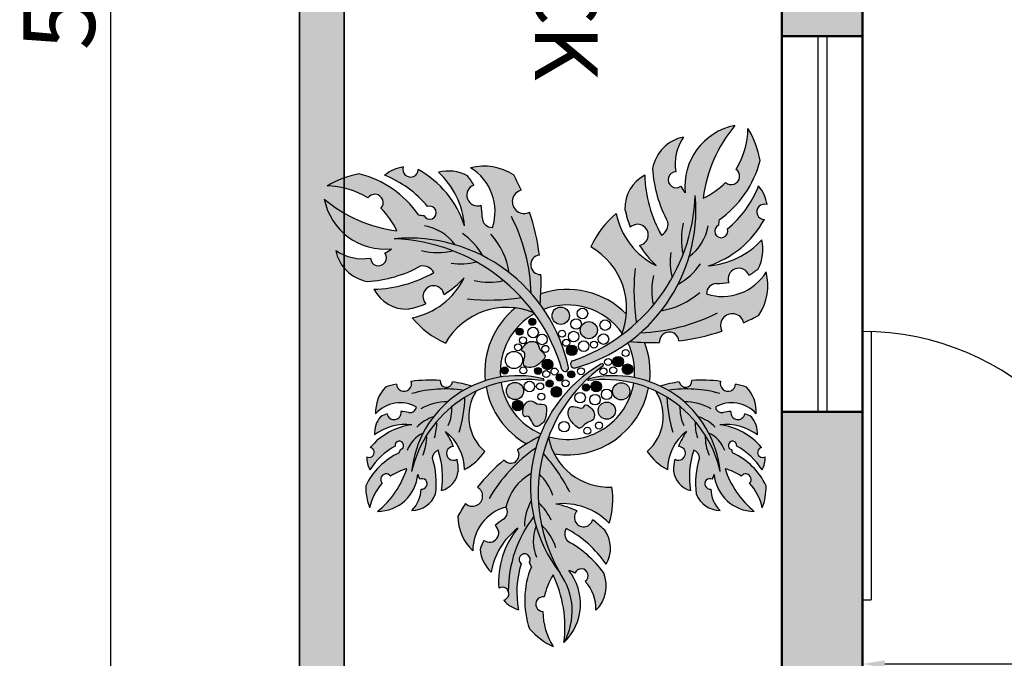
# Model space of a CAD drawing. Units: inches. Extents: x 3008 to 4088, y 1255 to 2137.
# Tile 4 of 30: x 3008 to 3119, y 1598 to 1670. Entities that reach past the tile are written whole.
import ezdxf

# ---------------------------------------------------------------- set-up
doc = ezdxf.new("R2010")
doc.units = ezdxf.units.IN
for name, color, linetype, lineweight in [('A-ANNO-DIMS', 2, 'Continuous', 18), ('A-ANNO-TEXT', 7, 'Continuous', 18), ('A-DOOR', 4, 'Continuous', 25), ('A-GLAZ', 4, 'Continuous', 25), ('A-WALL', 7, 'Continuous', 50), ('A-WALL-PATT', 8, 'Continuous', 13), ('C-PROP', 1, 'Continuous', 35), ('C-PROP-PATT', 9, 'Continuous', 13), ('estofado', 7, 'Continuous', 25), ('L-PLNT', 3, 'Continuous', 13)]:
    doc.layers.add(name, color=color, linetype=linetype, lineweight=lineweight)
doc.styles.get("Standard").update_dxf_attribs({"font": 'arial.ttf'})
doc.dimstyles.new('ISO-25', dxfattribs={"dimtxt": 8, "dimasz": 2.5, "dimexe": 1.25, "dimexo": 0.625, "dimtad": 1, "dimdec": 1, "dimlunit": 3, "dimtxsty": 'Standard', "dimcen": 2.5, "dimadec": 0, "dimazin": 0, "dimtfac": 1, "dimtdec": 1, "dimtmove": 0, "dimatfit": 3, "dimfxl": 1, "dimarcsym": 0})

# ---------------------------------------------------------------- blocks, each defined once
blk = doc.blocks.new('*D2')
at = {"layer": 'A-ANNO-DIMS', "color": 0, "lineweight": -2, "transparency": 16777216}
for p, q in [((3039.04, 2003.97), (3017.26, 2003.97)), ((3018.51, 2001.47), (3018.51, 1346.47)), ((3039.04, 1343.97), (3017.26, 1343.97))]:
    blk.add_line(p, q, dxfattribs=at)
at = {"layer": 'A-ANNO-DIMS', "color": 0, "transparency": 16777216}
for points in [[(3018.09, 2001.47), (3018.93, 2001.47), (3018.51, 2003.97)], [(3018.09, 1346.47), (3018.93, 1346.47), (3018.51, 1343.97)]]:
    blk.add_solid(points, dxfattribs=at)
at = {"layer": 'Defpoints', "color": 0, "transparency": 16777216}
for p in [(3039.67, 2003.97), (3018.51, 1343.97), (3039.67, 1343.97)]:
    blk.add_point(p, dxfattribs=at)
at = {"layer": 'A-ANNO-DIMS', "color": 0, "transparency": 16777216, "insert": (3013.82, 1673.97), "char_height": 8, "attachment_point": 5, "rotation": 90}
blk.add_mtext("55'", dxfattribs=at)
blk = doc.blocks.new('MD')
for p, q in [((1902.58, 1512.86), (1902.58, 1482.86)), ((1903.58, 1512.86), (1903.58, 1482.86)), ((1949.58, 1482.86), (1949.58, 1500.86)), ((1950.58, 1482.86), (1950.58, 1500.86)), ((1902.58, 1482.86), (1903.58, 1482.86)), ((1949.58, 1482.86), (1950.58, 1482.86))]:
    blk.add_line(p, q)
for centre, radius, start, end in [((1902.58, 1482.86), 30, 0, 90), ((1950.58, 1482.86), 18, 90, 180)]:
    blk.add_arc(centre, radius, start, end)
blk = doc.blocks.new('Novo Cashepo')
at = {"layer": 'estofado', "ltscale": 0.1}
h = blk.add_hatch(color=256, dxfattribs=at)
h.set_gradient(color1=(108, 164, 86), color2=(79, 120, 63), one_color=1, tint=0.36, name='CYLINDER')
h.paths.add_polyline_path([(0.2827, 0.4266, -0.314907), (0.2643, 0.3891, -0.122145), (0.2167, 0.5593, 0.291545), (0.1604, 0.4626, 0.043027), (0.1756, 0.4118, -1.339402), (0.202, 0.3602, 0.060072), (0.2488, 0.3031, -0.231117), (0.1355, 0.4506, 0.11449), (0.0635, 0.3561, -0.376746), (0.1502, 0.1049, 0.228124), (0.3602, 0.5016, -0.2613), (0.1736, 0.0872, 0.033062), (0.2588, 0.0848, -0.981895), (0.3134, 0.0893, 0.048855), (0.4361, 0.1168, -1.138233), (0.4978, 0.1407, 0.018864), (0.5414, 0.1623, 0.208979), (0.5618, 0.2847, -0.346636), (0.3922, 0.2224, -0.42625), (0.4225, 0.2519, 0.04537), (0.4552, 0.2547, -0.994855), (0.5125, 0.2753, 0.044381), (0.539, 0.2936, 0.18118), (0.5496, 0.3761, -0.18833), (0.3972, 0.3019, 0.191426), (0.5567, 0.4338, -1.174476), (0.5643, 0.4761, 0.140528), (0.5404, 0.529, -0.125367), (0.4517, 0.4068, -2.245001), (0.4262, 0.4175, -0.031976), (0.4282, 0.4328, 0.181425), (0.5443, 0.6013, 0.094503), (0.51, 0.6925, -0.138196), (0.476, 0.5769, -1.074478), (0.4463, 0.5393, -0.088291), (0.3828, 0.4942, -0.144087), (0.473, 0.7006, 0.388768), (0.3315, 0.5094, -0.041945), (0.3192, 0.5282, -1.340573), (0.3051, 0.5692, -0.196063), (0.327, 0.668, 0.307628), (0.2389, 0.5784, 0.111291)])
h = blk.add_hatch(color=256, dxfattribs=at)
h.set_gradient(color1=(108, 164, 86), color2=(102, 154, 81), one_color=1, tint=0.46, name='CYLINDER')
h.paths.add_polyline_path([(-0.0809, 0.1926, 0.033062), (-0.0785, 0.2778, -0.981895), (-0.0829, 0.3324, 0.048855), (-0.1105, 0.4551, -1.138233), (-0.1344, 0.5168, 0.018864), (-0.1559, 0.5604, 0.208979), (-0.2783, 0.5808, -0.346636), (-0.2161, 0.4112, -0.42625), (-0.2455, 0.4415, 0.04537), (-0.2484, 0.4742, -0.994855), (-0.269, 0.5315, 0.044381), (-0.2872, 0.5579, 0.18118), (-0.3697, 0.5686, -0.18833), (-0.2956, 0.4161, 0.191426), (-0.4275, 0.5757, -1.174476), (-0.4698, 0.5832, 0.140528), (-0.5227, 0.5593, -0.125367), (-0.4005, 0.4706, -2.245001), (-0.4112, 0.4452, -0.031976), (-0.4264, 0.4471, 0.181425), (-0.595, 0.5633, 0.094503), (-0.6862, 0.529, -0.138196), (-0.5706, 0.495, -1.074478), (-0.5329, 0.4652, -0.088291), (-0.4878, 0.4018, -0.144087), (-0.6943, 0.4919, 0.388768), (-0.503, 0.3504, -0.041945), (-0.5218, 0.3381, -1.340573), (-0.5628, 0.324, -0.196063), (-0.6617, 0.346, 0.307628), (-0.5721, 0.2579, 0.111291), (-0.4203, 0.3017, -0.314907), (-0.3828, 0.2833, -0.122145), (-0.553, 0.2356, 0.291545), (-0.4562, 0.1793, 0.043027), (-0.4055, 0.1946, -1.339402), (-0.3539, 0.2209, 0.060072), (-0.2968, 0.2677, -0.231117), (-0.4442, 0.1544, 0.11449), (-0.3498, 0.0824, -0.376746), (-0.0985, 0.1691, 0.228124), (-0.4952, 0.3792, -0.2613)])
h = blk.add_hatch(color=256, dxfattribs=at)
h.set_gradient(color1=(166, 115, 84), color2=(109, 75, 55), one_color=1, tint=0.32, name='INVCYLINDER')
h.paths.add_polyline_path([(0.3602, 0.5016, -0.309503), (0.0116, 0.0322, 0.812635), (0.0173, 0.012, 0.364481)])
h = blk.add_hatch(color=256, dxfattribs=at)
h.set_gradient(color1=(166, 115, 84), color2=(109, 75, 55), one_color=1, tint=0.32, name='INVCYLINDER')
h.paths.add_polyline_path([(-0.0186, 0.0079, 0.872708), (-0.0001, 0.0132, 0.378997), (-0.4952, 0.3792, -0.322151)])
h = blk.add_hatch(color=256, dxfattribs=at)
h.set_gradient(color1=(185, 193, 193), color2=(81, 92, 92), one_color=1, tint=0.34, name='CURVED')
h.paths.add_polyline_path([(0.1525, 0.1108, 0.06904), (0.1645, 0.1649, 0.288006), (-0.0787, 0.2226, -0.011646), (-0.0809, 0.1926, -0.009266), (-0.0709, 0.1786, -0.341204)])
h = blk.add_hatch(color=256, dxfattribs=at)
h.set_gradient(color1=(185, 193, 193), color2=(81, 92, 92), one_color=1, tint=0.34, name='CURVED')
h.paths.add_polyline_path([(-0.0966, 0.1665, 0.00155), (-0.0985, 0.1691, 0.067559), (-0.151, 0.1827, 0.253608), (-0.2368, -0.0242, -0.036817), (-0.1935, -0.0138, -0.290631)])
h = blk.add_hatch(color=256, dxfattribs=at)
h.set_gradient(color1=(179, 165, 128), color2=(150, 134, 90), one_color=1, tint=0.47)
h.paths.add_polyline_path([(-0.0466, 0.1604, -1), (0.0024, 0.1604, -1)])
h = blk.add_hatch(color=256, dxfattribs=at)
h.set_gradient(color1=(179, 165, 128), color2=(150, 134, 90), one_color=1, tint=0.47)
h.paths.add_polyline_path([(-0.113, 0.1431, 1), (-0.0932, 0.1431, 1)])
h = blk.add_hatch(color=256, dxfattribs=at)
h.set_gradient(color1=(179, 165, 128), color2=(150, 134, 90), one_color=1, tint=0.47)
h.paths.add_polyline_path([(0.0333, 0.1194, 1), (0.0824, 0.1194, 1)])
h = blk.add_hatch(color=256, dxfattribs=at)
h.set_gradient(color1=(179, 165, 128), color2=(150, 134, 90), one_color=1, tint=0.47)
h.paths.add_polyline_path([(-0.149, 0.1152, 1), (-0.1291, 0.1152, 1)])
h = blk.add_hatch(color=256, dxfattribs=at)
h.set_gradient(color1=(179, 165, 128), color2=(150, 134, 90), one_color=1, tint=0.47)
edge = h.paths.add_edge_path()
edge.add_spline(control_points=[(-0.126, 0.0391), (-0.128, 0.0314), (-0.132, 0.0156), (-0.099, 0.0101), (-0.0817, 0.025), (-0.0594, 0.0483), (-0.0851, 0.062), (-0.0856, 0.0869), (-0.1113, 0.0892), (-0.1235, 0.079), (-0.1379, 0.0613), (-0.1214, 0.0568), (-0.124, 0.0467), (-0.126, 0.0391)], knot_values=[0, 0, 0, 0, 0.020201, 0.040881, 0.075874, 0.093984, 0.117931, 0.138882, 0.158108, 0.177537, 0.194687, 0.200618, 0.219249, 0.219249, 0.219249, 0.219249], degree=3, periodic=0)
h = blk.add_hatch(color=256, dxfattribs=at)
h.set_gradient(color1=(185, 193, 193), color2=(81, 92, 92), one_color=1, tint=0.34, name='CURVED')
h.paths.add_polyline_path([(0.1736, 0.0872, -0.003321), (0.1687, 0.0836, -0.134103), (0.1873, -0.0153, -0.036923), (0.2304, -0.0269, 0.121396), (0.2162, 0.0846, -0.016535)])
h = blk.add_hatch(color=256, dxfattribs=at)
h.set_gradient(color1=(179, 165, 128), color2=(150, 134, 90), one_color=1, tint=0.47)
h.paths.add_polyline_path([(0.0244, 0.0622, 1), (-0.0057, 0.0622, 1)])
h = blk.add_hatch(color=256, dxfattribs=at)
h.set_gradient(color1=(179, 165, 128), color2=(150, 134, 90), one_color=1, tint=0.47)
h.paths.add_polyline_path([(-0.0448, 0.022, 1), (-0.0748, 0.022, 1)])
h = blk.add_hatch(color=256, dxfattribs=at)
h.set_gradient(color1=(179, 165, 128), color2=(150, 134, 90), one_color=1, tint=0.47)
h.paths.add_polyline_path([(0.1562, 0.0298, 1), (0.1262, 0.0298, 1)])
h = blk.add_hatch(color=256, dxfattribs=at)
h.set_gradient(color1=(179, 165, 128), color2=(150, 134, 90), one_color=1, tint=0.47)
h.paths.add_polyline_path([(-0.1713, 0.0047, 1), (-0.1912, 0.0047, 1)])
h = blk.add_hatch(color=256, dxfattribs=at)
h.set_gradient(color1=(166, 115, 84), color2=(109, 75, 55), one_color=1, tint=0.32, name='INVCYLINDER')
h.paths.add_polyline_path([(0.0994, 0.0192, 0.726279), (0.0923, 0.0227, 0.000011), (0.0923, 0.0227, 0.454782), (-0.024, -0.5707, -0.387777)])
h = blk.add_hatch(color=256, dxfattribs=at)
h.set_gradient(color1=(179, 165, 128), color2=(150, 134, 90), one_color=1, tint=0.47)
h.paths.add_polyline_path([(-0.0766, 0.0036, 1), (-0.0965, 0.0036, 1)])
h = blk.add_hatch(color=256, dxfattribs=at)
h.set_gradient(color1=(179, 165, 128), color2=(150, 134, 90), one_color=1, tint=0.47)
h.paths.add_polyline_path([(0.0176, -0.0063, 1), (-0.0023, -0.0063, 1)])
h = blk.add_hatch(color=256, dxfattribs=at)
h.set_gradient(color1=(179, 165, 128), color2=(150, 134, 90), one_color=1, tint=0.47)
h.paths.add_polyline_path([(0.1828, 0.0084, 1), (0.1527, 0.0084, 1)])
h = blk.add_hatch(color=256, dxfattribs=at)
h.set_gradient(color1=(108, 164, 86), color2=(62, 94, 49), one_color=1, tint=0.28, name='CURVED')
h.paths.add_polyline_path([(-0.5633, -0.214, -1.174476), (-0.5734, -0.2402, 0.140528), (-0.5646, -0.277, -0.125367), (-0.4927, -0.2097, -2.245001), (-0.4777, -0.2197, -0.031976), (-0.4809, -0.2292, 0.181425), (-0.5761, -0.3228, 0.094503), (-0.5654, -0.3855, -0.138196), (-0.5293, -0.3156, -1.074478), (-0.5056, -0.2952, -0.088291), (-0.4594, -0.2742, -0.144087), (-0.5427, -0.3952, 0.388768), (-0.4284, -0.2902, -0.041945), (-0.4229, -0.3038, -1.340573), (-0.4189, -0.3318, -0.196063), (-0.4452, -0.3924, 0.307628), (-0.3777, -0.3459, 0.111291), (-0.387, -0.2433, -0.314907), (-0.3706, -0.2216, -0.122145), (-0.3611, -0.3364, 0.291545), (-0.3131, -0.2814, 0.043027), (-0.3166, -0.247, -1.339402), (-0.3271, -0.2108, 0.060072), (-0.35, -0.1684, -0.231117), (-0.2957, -0.2768, 0.11449), (-0.2379, -0.2252, -0.376746), (-0.2623, -0.0537, 0.228124), (-0.4459, -0.2817, -0.2613), (-0.2752, -0.0394, 0.033062), (-0.3295, -0.0274, -0.981895), (-0.365, -0.0235, 0.048855), (-0.4469, -0.026, -1.138233), (-0.4894, -0.0336, 0.018864), (-0.52, -0.042, 0.208979), (-0.5481, -0.1179, -0.346636), (-0.4319, -0.099, -0.42625), (-0.4549, -0.1141, 0.04537), (-0.4762, -0.1119, -0.994855), (-0.5154, -0.118, 0.044381), (-0.5346, -0.1264, 0.18118), (-0.5516, -0.1779, -0.18833), (-0.4449, -0.1493, 0.191426)])
h = blk.add_hatch(color=256, dxfattribs=at)
h.set_gradient(color1=(166, 115, 84), color2=(109, 75, 55), one_color=1, tint=0.32, name='INVCYLINDER')
h.paths.add_polyline_path([(-0.0708, -0.0241, 0.529291), (-0.0712, -0.0189, 0.456534), (-0.4459, -0.2817, -0.387777)])
h = blk.add_hatch(color=256, dxfattribs=at)
h.set_gradient(color1=(179, 165, 128), color2=(150, 134, 90), one_color=1, tint=0.47)
h.paths.add_polyline_path([(-0.0439, -0.0322, 1), (-0.0638, -0.0322, 1)])
h = blk.add_hatch(color=256, dxfattribs=at)
h.set_gradient(color1=(179, 165, 128), color2=(150, 134, 90), one_color=1, tint=0.47)
h.paths.add_polyline_path([(-0.0152, -0.0149, 1), (-0.0351, -0.0149, 1)])
h = blk.add_hatch(color=256, dxfattribs=at)
h.set_gradient(color1=(166, 115, 84), color2=(109, 75, 55), one_color=1, tint=0.32, name='INVCYLINDER')
h.paths.add_polyline_path([(0.4314, -0.2817, 0.456534), (0.0566, -0.0189, 0.529291), (0.0563, -0.0241, -0.387777)])
h = blk.add_hatch(color=256, dxfattribs=at)
h.set_gradient(color1=(179, 165, 128), color2=(150, 134, 90), one_color=1, tint=0.47)
h.paths.add_polyline_path([(0.0939, -0.0406, 1), (0.0639, -0.0406, 1)])
h = blk.add_hatch(color=256, dxfattribs=at)
h.set_gradient(color1=(108, 164, 86), color2=(154, 193, 138), one_color=1, tint=0.65, name='HEMISPHERICAL')
h.paths.add_polyline_path([(0.4174, -0.099, -0.346636), (0.5336, -0.1179, 0.208979), (0.5055, -0.042, 0.018864), (0.4749, -0.0336, -1.138233), (0.4324, -0.026, 0.048855), (0.3504, -0.0235, -0.981895), (0.3149, -0.0274, 0.033062), (0.2607, -0.0394, -0.2613), (0.4314, -0.2817, 0.228124), (0.2478, -0.0537, -0.376746), (0.2234, -0.2252, 0.11449), (0.2812, -0.2768, -0.231117), (0.3355, -0.1684, 0.060072), (0.3126, -0.2108, -1.339402), (0.3021, -0.247, 0.043027), (0.2986, -0.2814, 0.291545), (0.3466, -0.3364, -0.122145), (0.3561, -0.2216, -0.314907), (0.3725, -0.2433, 0.111291), (0.3632, -0.3459, 0.307628), (0.4307, -0.3924, -0.196063), (0.4044, -0.3318, -1.340573), (0.4084, -0.3038, -0.041945), (0.4139, -0.2902, 0.388768), (0.5282, -0.3952, -0.144087), (0.4449, -0.2742, -0.088291), (0.4911, -0.2952, -1.074478), (0.5148, -0.3156, -0.138196), (0.5509, -0.3855, 0.094503), (0.5616, -0.3228, 0.181425), (0.4664, -0.2292, -0.031976), (0.4632, -0.2197, -2.245001), (0.4782, -0.2097, -0.125367), (0.5501, -0.277, 0.140528), (0.5589, -0.2402, -1.174476), (0.5488, -0.214, 0.191426), (0.4304, -0.1493, -0.18833), (0.5371, -0.1779, 0.18118), (0.5201, -0.1264, 0.044381), (0.5009, -0.118, -0.994855), (0.4617, -0.1119, 0.04537), (0.4404, -0.1141, -0.42625)])
h = blk.add_hatch(color=256, dxfattribs=at)
h.set_gradient(color1=(185, 193, 193), color2=(81, 92, 92), one_color=1, tint=0.34, name='CURVED')
h.paths.add_polyline_path([(-0.1917, -0.0292, 0.03292), (-0.2343, -0.0418, 0.221446), (-0.1198, -0.2039, -0.019377), (-0.0822, -0.1825, -0.005069), (-0.0793, -0.175, -0.256969)])
h = blk.add_hatch(color=256, dxfattribs=at)
h.set_gradient(color1=(179, 165, 128), color2=(150, 134, 90), one_color=1, tint=0.47)
h.paths.add_polyline_path([(-0.1275, -0.0533, 1), (-0.1765, -0.0533, 1)])
h = blk.add_hatch(color=256, dxfattribs=at)
h.set_gradient(color1=(185, 193, 193), color2=(81, 92, 92), one_color=1, tint=0.34, name='CURVED')
h.paths.add_polyline_path([(0.1853, -0.0311, -0.449638), (-0.0565, -0.1832, 0.000699), (-0.0569, -0.1844, 0.072477), (-0.0408, -0.2319, 0.40511), (0.2276, -0.0448, 0.032975)])
h = blk.add_hatch(color=256, dxfattribs=at)
h.set_gradient(color1=(179, 165, 128), color2=(150, 134, 90), one_color=1, tint=0.47)
h.paths.add_polyline_path([(-0.0194, -0.0559, 1), (-0.0495, -0.0559, 1)])
h = blk.add_hatch(color=256, dxfattribs=at)
h.set_gradient(color1=(179, 165, 128), color2=(150, 134, 90), one_color=1, tint=0.47)
h.paths.add_polyline_path([(0.0597, -0.0435, 1), (0.0398, -0.0435, 1)])
h = blk.add_hatch(color=256, dxfattribs=at)
h.set_gradient(color1=(179, 165, 128), color2=(150, 134, 90), one_color=1, tint=0.47)
h.paths.add_polyline_path([(0.1743, -0.0543, 1), (0.1253, -0.0543, 1)])
h = blk.add_hatch(color=256, dxfattribs=at)
h.set_gradient(color1=(179, 165, 128), color2=(150, 134, 90), one_color=1, tint=0.47)
h.paths.add_polyline_path([(-0.1294, -0.0948, 1), (-0.1594, -0.0948, 1)])
h = blk.add_hatch(color=256, dxfattribs=at)
h.set_gradient(color1=(179, 165, 128), color2=(150, 134, 90), one_color=1, tint=0.47)
edge = h.paths.add_edge_path()
edge.add_spline(control_points=[(-0.1055, -0.1384), (-0.1019, -0.1456), (-0.0945, -0.16), (-0.0661, -0.1423), (-0.063, -0.1197), (-0.0617, -0.0875), (-0.09, -0.0942), (-0.1068, -0.0758), (-0.1276, -0.0911), (-0.13, -0.1069), (-0.1291, -0.1297), (-0.1137, -0.1221), (-0.1091, -0.1314), (-0.1055, -0.1384)], knot_values=[0, 0, 0, 0, 0.020201, 0.040881, 0.075874, 0.093984, 0.117931, 0.138882, 0.158108, 0.177537, 0.194687, 0.200618, 0.219249, 0.219249, 0.219249, 0.219249], degree=3, periodic=0)
h = blk.add_hatch(color=256, dxfattribs=at)
h.set_gradient(color1=(179, 165, 128), color2=(150, 134, 90), one_color=1, tint=0.47)
edge = h.paths.add_edge_path()
edge.add_spline(control_points=[(0.0251, -0.0997), (0.0173, -0.0977), (0.0016, -0.0937), (-0.004, -0.1268), (0.011, -0.1441), (0.0343, -0.1664), (0.0479, -0.1407), (0.0728, -0.1402), (0.0751, -0.1145), (0.0649, -0.1023), (0.0473, -0.0879), (0.0427, -0.1044), (0.0327, -0.1017), (0.0251, -0.0997)], knot_values=[0, 0, 0, 0, 0.020201, 0.040881, 0.075874, 0.093984, 0.117931, 0.138882, 0.158108, 0.177537, 0.194687, 0.200618, 0.219249, 0.219249, 0.219249, 0.219249], degree=3, periodic=0)
h = blk.add_hatch(color=256, dxfattribs=at)
h.set_gradient(color1=(179, 165, 128), color2=(150, 134, 90), one_color=1, tint=0.47)
h.paths.add_polyline_path([(0.1333, -0.1092, 1), (0.0843, -0.1092, 1)])
h = blk.add_hatch(color=256, dxfattribs=at)
h.set_gradient(color1=(108, 164, 86), color2=(128, 178, 108), one_color=1, tint=0.56, name='CYLINDER')
h.paths.add_polyline_path([(-0.0931, -0.2153, -0.021499), (-0.0822, -0.1825, 0.033062), (-0.1452, -0.2207, -0.981895), (-0.1828, -0.2494, 0.048855), (-0.259, -0.3268, -1.138233), (-0.2927, -0.373, 0.018864), (-0.3143, -0.409, 0.208979), (-0.2718, -0.5074, -0.346636), (-0.1778, -0.383, -0.218356), (-0.1066, -0.288, -0.045186), (-0.0935, -0.2168, -0.00127), (-0.0946, -0.2163, -0.001036)])
h = blk.add_hatch(color=256, dxfattribs=at)
h.set_gradient(color1=(108, 164, 86), color2=(128, 178, 108), one_color=1, tint=0.56, name='CYLINDER')
h.paths.add_polyline_path([(0.1153, -0.4286, 0.11449), (0.1235, -0.3263, -0.376746), (-0.0569, -0.1844, 0.228124), (-0.024, -0.5707, -0.289779), (-0.0128, -0.768, 0.388768), (0.0005, -0.5629, -0.041945), (0.0182, -0.5708, -1.340573), (0.0477, -0.594, -0.196063), (0.0779, -0.676, 0.307628), (0.1, -0.5698, 0.111291), (-0.0028, -0.48, -0.314907), (-0.0069, -0.4442, -0.122145), (0.1072, -0.5455, 0.291545), (0.1029, -0.4489, 0.043027), (0.0681, -0.4192, -1.339402), (0.0248, -0.3941, 0.060072), (-0.0358, -0.3745, -0.231117)])
h = blk.add_hatch(color=256, dxfattribs=at)
h.set_gradient(color1=(108, 164, 86), color2=(128, 178, 108), one_color=1, tint=0.56, name='CYLINDER')
h.paths.add_polyline_path([(-0.186, -0.4185, 0.04537), (-0.2084, -0.4358, -0.994855), (-0.2404, -0.4776, 0.044381), (-0.2511, -0.5032, 0.18118), (-0.2202, -0.5681, -0.18833), (-0.1442, -0.443, 0.191426), (-0.1984, -0.6134, -0.461932), (-0.1711, -0.6221, -0.164855), (-0.099, -0.4106, -0.076989), (-0.1066, -0.288, 0.218356), (-0.1778, -0.383, -0.42625)])
h = blk.add_hatch(color=256, dxfattribs=at)
h.set_gradient(color1=(108, 164, 86), color2=(128, 178, 108), one_color=1, tint=0.56, name='CYLINDER')
h.paths.add_polyline_path([(-0.1111, -0.7292, 0.094503), (-0.0435, -0.7794, -0.138196), (-0.0729, -0.6796, -1.074478), (-0.0689, -0.6383, -0.088291), (-0.0439, -0.5759, -0.144087), (-0.0128, -0.768, 0.289779), (-0.024, -0.5707, -0.111568), (-0.099, -0.4106, 0.164855), (-0.1711, -0.6221, -0.461932), (-0.1841, -0.6476, 0.140528), (-0.142, -0.6749, -0.125367), (-0.1347, -0.5446, -2.245001), (-0.1112, -0.5405, -0.031976), (-0.1055, -0.5525, 0.181425)])
for centre, radius in [((-0.0221, 0.1604), 0.0245), ((0.0395, 0.1667), 0.015), ((-0.1031, 0.1431), 0.00994), ((0.0215, 0.1368), 0.015), ((0.0578, 0.1194), 0.0245), ((0.1044, 0.1338), 0.015), ((-0.1391, 0.1152), 0.00994), ((-0.1006, 0.1127), 0.015), ((-0.0182, 0.1092), 0.00994), ((0.0145, 0.1013), 0.015), ((-0.1296, 0.0906), 0.00994), ((-0.0753, 0.0931), 0.015), ((-0.0066, 0.0836), 0.00994), ((0.0432, 0.0739), 0.015), ((0.0724, 0.0784), 0.00994), ((0.0993, 0.0941), 0.015), ((-0.155, 0.0346), 0.0245), ((-0.1435, 0.0709), 0.00994), ((-0.0657, 0.0663), 0.00994), ((0.0093, 0.0622), 0.015), ((0.1627, 0.0543), 0.00994), ((-0.0598, 0.022), 0.015), ((0.1127, 0.0289), 0.00994), ((0.1412, 0.0298), 0.015), ((-0.1813, 0.0047), 0.00994), ((-0.1282, 0.0051), 0.00994), ((-0.0866, 0.0036), 0.00994), ((-0.0635, -0.0053), 0.00994), ((-0.0398, 0.002), 0.00994), ((0.0077, -0.0063), 0.00994), ((0.0352, 0.0026), 0.00994), ((0.0994, 0.0024), 0.00994), ((0.127, 0.0055), 0.00994), ((0.1678, 0.0084), 0.015), ((-0.1111, -0.0406), 0.015), ((-0.0539, -0.0322), 0.00994), ((-0.0252, -0.0149), 0.00994), ((-0.0085, -0.0314), 0.00994), ((0.0789, -0.0406), 0.015), ((-0.152, -0.0533), 0.0245), ((-0.0806, -0.0403), 0.00994), ((-0.0345, -0.0559), 0.015), ((0.0498, -0.0435), 0.00994), ((0.1084, -0.0629), 0.015), ((0.1498, -0.0543), 0.0245), ((-0.1444, -0.0948), 0.015), ((-0.0774, -0.0694), 0.00994), ((0.0329, -0.0722), 0.015), ((0.0754, -0.0779), 0.015), ((0.1088, -0.1092), 0.0245), ((-0.0125, -0.1547), 0.015), ((0.0538, -0.1663), 0.00994), ((0.0867, -0.1514), 0.00994)]:
    blk.add_circle(centre, radius, dxfattribs=at)
for centre, radius, start, end in [((0.5066, 0.5278), 0.1761, 101.0186, 185.9966), ((0.7787, 0.4442), 0.399, 140.0122, 172.8088), ((0.2879, 0.6951), 0.2222, 327.8752, 359.3481), ((0.2881, 0.557), 0.26, 9.8207, 31.4151), ((0.3489, 0.5584), 0.1118, 101.2825, 169.6799), ((0.4372, 0.5917), 0.134, 145.305, 189.6765), ((0.2616, 0.6719), 0.2914, 304.8613, 345.9935), ((-0.5506, 0.307), 0.26, 99.8207, 121.4151), ((-0.6655, 0.2806), 0.2914, 34.8613, 75.9935), ((-0.4545, 0.479), 0.1053, 98.3059, 130.3029), ((-0.4492, 0.576), 0.0218, 160.6631, 359.0131), ((-0.5622, 0.33), 0.2802, 17.9062, 61.2534), ((-0.3427, 0.4531), 0.1185, 62.1153, 103.1932), ((-0.5278, 0.3974), 0.233, 4.6076, 47.2701), ((-0.2404, 0.4305), 0.1549, 56.9429, 104.1578), ((-0.3548, 0.4565), 0.1459, 341.9118, 58.3844), ((-0.7231, 0.2531), 0.6451, 24.1234, 28.4463), ((0.5976, 0.5997), 0.3593, 183.393, 208.7944), ((0.306, 0.5466), 0.0226, 92.4292, 305.5449), ((0.4625, 0.557), 0.024, 227.5673, 55.7919), ((-0.6357, 0.2751), 0.3059, 39.7257, 68.3087), ((-0.4269, 0.4422), 0.1813, 29.481, 39.6456), ((0.2645, 0.4667), 0.1042, 117.2921, 182.3073), ((0.5836, 0.5703), 0.3671, 181.7055, 209.5612), ((0.2879, 0.6951), 0.2222, 295.3016, 315.484), ((-0.6887, 0.3068), 0.2222, 57.8752, 89.3481), ((-0.5507, 0.4815), 0.024, 317.5673, 145.7919), ((-0.2585, 0.5029), 0.0304, 110.1108, 289.5198), ((-0.1264, 0.4844), 0.0334, 103.7865, 298.5822), ((0.4372, 0.5917), 0.134, 208.2976, 217.9049), ((0.2562, 0.6421), 0.3059, 309.7257, 338.3087), ((0.4601, 0.4609), 0.1053, 8.3059, 40.3029), ((-0.4379, 0.7976), 0.399, 230.0122, 262.8088), ((-0.5214, 0.5256), 0.1761, 191.0186, 275.9966), ((-0.1569, 0.5215), 0.5175, 289.0066, 357.7964), ((-0.1024, 0.4607), 0.4645, 284.942, 5.0453), ((0.5571, 0.4556), 0.0218, 70.6631, 269.0131), ((-0.6887, 0.3068), 0.2222, 25.3016, 45.484), ((-0.3944, 0.4531), 0.0186, 205.201, 109.1617), ((-0.4269, 0.4422), 0.1813, 359.2754, 10.1496), ((-0.7231, 0.2531), 0.6451, 7.0576, 18.2453), ((0.303, 0.2481), 0.2627, 129.608, 155.7334), ((0.3431, 0.4928), 0.2118, 191.5061, 243.5602), ((0.4622, 0.5257), 0.3083, 191.8137, 201.6687), ((-0.4035, 0.5652), 0.1203, 259.0186, 266.3445), ((-0.2163, 0.4404), 0.0293, 181.0153, 270.3634), ((-0.6263, 0.2061), 0.5206, 1.9256, 26.9542), ((0.1964, 0.3899), 0.0302, 280.5489, 133.5686), ((0.2467, 0.421), 0.0364, 298.8789, 8.7972), ((0.5076, 0.3784), 0.1869, 165.9423, 193.4167), ((0.311, 0.5686), 0.2802, 287.9062, 331.2534), ((0.5463, 0.4099), 0.1203, 169.0186, 176.3445), ((-0.4326, 0.2811), 0.1367, 36.1411, 80.3873), ((-0.4031, 0.2432), 0.1817, 28.6905, 56.0246), ((0.2622, 0.4389), 0.1367, 306.1411, 350.3873), ((0.4341, 0.4007), 0.0186, 115.201, 19.1617), ((-0.4544, -0.0835), 0.4645, 12.0191, 95.0453), ((-0.5151, -0.138), 0.5175, 16.3708, 87.7964), ((-0.3847, 0.2462), 0.2195, 9.4944, 41.5537), ((0.3785, 0.5342), 0.233, 274.6076, 317.2701), ((0.4342, 0.349), 0.1185, 332.1153, 13.1932), ((-0.5854, 0.4562), 0.134, 235.305, 279.6765), ((-0.5521, 0.3678), 0.1118, 191.2825, 259.6799), ((-0.5402, 0.325), 0.0226, 182.4292, 35.5449), ((-0.5854, 0.4562), 0.134, 298.2976, 307.9049), ((-0.372, 0.5266), 0.1869, 255.9423, 283.4167), ((-0.0362, 0.1811), 0.2014, 337.7465, 60.3213), ((0.4622, 0.5257), 0.3083, 212.4488, 226.1997), ((0.4824, 0.3139), 0.1936, 172.3137, 193.7119), ((-0.3076, 0.5014), 0.1936, 262.3137, 283.7119), ((-0.0802, 0.3051), 0.0274, 95.6708, 273.5772), ((0.2242, 0.4094), 0.1817, 298.6905, 326.0246), ((-0.5933, 0.6166), 0.3593, 273.393, 298.7944), ((-0.5639, 0.6026), 0.3671, 271.7055, 299.5612), ((-0.4147, 0.2657), 0.0364, 28.8789, 98.7972), ((0.8078, 0.234), 0.6217, 174.4084, 188.6615), ((0.4375, 0.3611), 0.1459, 251.9118, 328.3844), ((0.4839, 0.2649), 0.0304, 20.1108, 199.5198), ((0.4233, 0.4332), 0.1813, 299.481, 309.6456), ((0.4116, 0.2468), 0.1549, 326.9429, 14.1578), ((-0.4865, 0.362), 0.2118, 281.5061, 333.5602), ((-0.5193, 0.4811), 0.3083, 302.4488, 316.1997), ((-0.2254, 0.4264), 0.1711, 255.544, 283.8081), ((-0.7231, 0.2531), 0.6451, 354.6159, 2.1904), ((0.4075, 0.2318), 0.1711, 165.544, 193.8081), ((0.4215, 0.2226), 0.0293, 91.0153, 180.3634), ((0.4233, 0.4332), 0.1813, 269.2754, 280.1496), ((-0.4604, 0.2834), 0.1042, 207.2921, 272.3073), ((-0.3836, 0.2154), 0.0302, 10.5489, 223.5686), ((-0.003, 0.0001), 0.235, 44.5248, 108.7916), ((0.2272, 0.3911), 0.2195, 279.4944, 311.5537), ((-0.2276, 0.8267), 0.6217, 264.4084, 278.6615), ((-0.5193, 0.4811), 0.3083, 281.8137, 291.6687), ((-0.1748, -0.0173), 0.2014, 67.7465, 150.3213), ((-0.003, 0.0001), 0.235, 129.0122, 185.9347), ((-0.003, 0.0001), 0.1909, 35.4554, 110.8148), ((0.1872, 0.6326), 0.5206, 271.9256, 296.9542), ((-0.2418, 0.3219), 0.2627, 219.608, 245.7334), ((-0.003, 0.0001), 0.1909, 119.3518, 184.1737), ((0.4654, 0.1328), 0.0334, 13.7865, 208.5822), ((0.2342, 0.7294), 0.6451, 294.1234, 298.4463), ((0.2862, 0.0866), 0.0274, 5.6708, 183.5772), ((0.2342, 0.7294), 0.6451, 277.0576, 288.2453), ((0.2342, 0.7294), 0.6451, 264.6159, 272.1904), ((-0.003, 0.0001), 0.235, 353.3979, 21.0844), ((-0.003, 0.0001), 0.1909, 355.3819, 25.9338), ((0.0166, 0.0227), 0.0107, 117.5535, 273.9476), ((0.2929, -0.3247), 0.4012, 120.0005, 217.8213), ((0.3609, -0.3433), 0.447, 125.7916, 210.5723), ((-0.0097, 0.0118), 0.00971, 203.8853, 8.3312), ((0.0953, 0.0198), 0.00417, 352.069, 136.0321), ((-0.4677, -0.0325), 0.0217, 182.8615, 17.6572), ((-0.3933, -0.4432), 0.4207, 86.1325, 97.3203), ((-0.1446, -0.3127), 0.3029, 76.2995, 174.1203), ((-0.1172, -0.3583), 0.3375, 82.0906, 166.8713), ((-0.3472, -0.0251), 0.0179, 174.7458, 352.6522), ((-0.3933, -0.4432), 0.4207, 73.6909, 81.2654), ((-0.0727, -0.0216), 0.00315, 308.368, 92.3311), ((0.0582, -0.0216), 0.00315, 87.6689, 231.632), ((0.1027, -0.3583), 0.3375, 13.1287, 97.9094), ((0.1301, -0.3127), 0.3029, 5.8797, 103.7005), ((0.3788, -0.4432), 0.4207, 98.7346, 106.3091), ((0.3327, -0.0251), 0.0179, 187.3478, 5.2542), ((0.3788, -0.4432), 0.4207, 82.6797, 93.8675), ((0.4531, -0.0325), 0.0217, 162.3428, 357.1385), ((-0.4473, -0.1122), 0.101, 136.0179, 183.2328), ((-0.3933, -0.4432), 0.4207, 103.1984, 107.5212), ((-0.3513, -0.387), 0.3395, 81.0006, 106.0292), ((-0.1524, -0.1255), 0.1313, 146.8215, 229.3963), ((-0.003, 0.0001), 0.235, 190.2712, 240.2168), ((-0.003, 0.0001), 0.1909, 188.82, 246.4657), ((-0.003, 0.0001), 0.1909, 253.7485, 350.5904), ((-0.003, 0.0001), 0.235, 260.7676, 348.9809), ((0.1379, -0.1255), 0.1313, 310.6037, 33.1785), ((0.3368, -0.387), 0.3395, 73.9708, 98.9994), ((0.3788, -0.4432), 0.4207, 72.4788, 76.8016), ((0.4328, -0.1122), 0.101, 356.7672, 43.9821), ((-0.6994, -0.055), 0.4054, 343.4834, 357.7365), ((0.6849, -0.055), 0.4054, 182.2635, 196.5166), ((-0.478, -0.1822), 0.0952, 60.9868, 137.4594), ((-0.4958, -0.1149), 0.0199, 189.1858, 8.5947), ((-0.4778, -0.2301), 0.1183, 78.3504, 89.2246), ((-0.4506, -0.0955), 0.0191, 260.0903, 349.4383), ((-0.3471, -0.2274), 0.1431, 88.5693, 120.6287), ((-0.4428, -0.1031), 0.1116, 334.6189, 2.8831), ((0.4283, -0.1031), 0.1116, 177.1169, 205.3811), ((0.3325, -0.2274), 0.1431, 59.3713, 91.4307), ((0.4635, -0.1822), 0.0952, 42.5406, 119.0132), ((0.4361, -0.0955), 0.0191, 190.5617, 279.9097), ((0.4633, -0.2301), 0.1183, 90.7754, 101.6496), ((0.4813, -0.1149), 0.0199, 171.4053, 350.8142), ((-0.4744, -0.1749), 0.0773, 141.1903, 182.2681), ((-0.4778, -0.2301), 0.1183, 108.5559, 118.7205), ((-0.3474, -0.2395), 0.1185, 107.7654, 135.0996), ((0.3329, -0.2395), 0.1185, 44.9004, 72.2346), ((0.4633, -0.2301), 0.1183, 61.2795, 71.4441), ((0.4599, -0.1749), 0.0773, 357.7319, 38.8097), ((-0.4227, -0.3307), 0.1827, 96.9812, 140.3284), ((-0.4616, -0.3003), 0.1519, 83.6826, 126.345), ((-0.5009, -0.1464), 0.1263, 341.3887, 2.7869), ((0.4864, -0.1464), 0.1263, 177.2131, 198.6113), ((0.4471, -0.3003), 0.1519, 53.655, 96.3174), ((0.4082, -0.3307), 0.1827, 39.6716, 83.0188), ((-0.4807, -0.208), 0.0121, 284.2759, 188.2367), ((-0.3754, -0.2537), 0.0892, 115.216, 159.4623), ((-0.525, -0.1846), 0.1219, 335.0173, 2.4916), ((-0.5141, -0.2845), 0.2011, 21.5237, 35.2746), ((-0.4338, -0.2782), 0.1381, 0.581, 52.6352), ((0.1741, -0.6772), 0.5572, 117.3918, 124.9664), ((0.1141, -0.1526), 0.1739, 190.5225, 273.0973), ((0.4193, -0.2782), 0.1381, 127.3648, 179.419), ((0.4996, -0.2845), 0.2011, 144.7254, 158.4763), ((0.5105, -0.1846), 0.1219, 177.5084, 204.9827), ((0.3608, -0.2537), 0.0892, 20.5377, 64.784), ((0.4662, -0.208), 0.0121, 351.7633, 255.7241), ((-0.5662, -0.2279), 0.0142, 239.7381, 78.088), ((-0.3966, -0.3845), 0.1995, 118.8007, 147.3836), ((-0.5537, -0.2), 0.0785, 338.0936, 345.4195), ((-0.3633, -0.2442), 0.0238, 107.9539, 177.8722), ((-0.5974, -0.2981), 0.2394, 350.7805, 18.6362), ((-0.3272, -0.2305), 0.0197, 89.6239, 302.6435), ((0.1629, -0.585), 0.4497, 124.7016, 149.7302), ((-0.1643, -0.2347), 0.0237, 218.4468, 36.3532), ((-0.003, 0.0001), 0.235, 247.0716, 247.3627), ((0.3127, -0.2305), 0.0197, 237.3565, 90.3761), ((0.5829, -0.2981), 0.2394, 161.3638, 189.2195), ((0.3487, -0.2442), 0.0238, 2.1278, 72.0461), ((0.5392, -0.2), 0.0785, 194.5805, 201.9064), ((0.3821, -0.3845), 0.1995, 32.6164, 61.1993), ((0.5517, -0.2279), 0.0142, 101.912, 300.2619), ((-0.4038, -0.4029), 0.19, 113.9363, 155.0685), ((-0.5048, -0.2433), 0.0687, 177.3808, 209.3779), ((-0.61, -0.3152), 0.2343, 352.4679, 17.8694), ((-0.5141, -0.2845), 0.2011, 0.8887, 10.7437), ((-0.3779, -0.1265), 0.1713, 298.683, 324.8084), ((0.1741, -0.6772), 0.5572, 129.8335, 141.0213), ((-0.4741, -0.5856), 0.5369, 27.1843, 41.4375), ((0.3634, -0.1265), 0.1713, 215.1916, 241.317), ((0.4996, -0.2845), 0.2011, 169.2563, 179.1113), ((0.5955, -0.3152), 0.2343, 162.1306, 187.5321), ((0.3893, -0.4029), 0.19, 24.9315, 66.0637), ((0.4903, -0.2433), 0.0687, 330.6221, 2.6192), ((-0.7067, -0.1933), 0.2602, 309.0872, 341.8838), ((-0.4235, -0.4145), 0.1449, 104.3766, 124.559), ((0.4089, -0.4145), 0.1449, 55.441, 75.6234), ((0.6922, -0.1933), 0.2602, 198.1162, 230.9128), ((-0.5429, -0.2804), 0.1149, 270.0936, 355.0715), ((-0.5182, -0.3046), 0.0157, 36.6423, 224.8669), ((-0.5063, -0.3299), 0.0874, 17.3725, 26.9799), ((-0.4167, -0.3172), 0.0148, 261.5041, 114.6198), ((-0.3803, -0.2712), 0.0679, 286.3671, 351.3823), ((-0.0386, -0.4131), 0.1424, 118.5185, 167.7887), ((-0.1845, -0.3969), 0.1478, 18.3199, 46.584), ((0.3657, -0.2712), 0.0679, 188.6177, 253.6329), ((0.4022, -0.3172), 0.0148, 65.3802, 278.4959), ((0.4918, -0.3299), 0.0874, 153.0201, 162.6275), ((0.5283, -0.2804), 0.1149, 184.9285, 269.9064), ((0.5037, -0.3046), 0.0157, 315.1331, 143.3577), ((-0.4065, -0.3261), 0.1696, 178.8957, 200.49), ((-0.4235, -0.4145), 0.1449, 136.9502, 168.4231), ((-0.5063, -0.3299), 0.0874, 314.38, 358.7514), ((-0.2728, -0.352), 0.0288, 226.5625, 61.3582), ((-0.1009, -0.3599), 0.2269, 342.384, 8.5094), ((0.4918, -0.3299), 0.0874, 181.2486, 225.62), ((0.4089, -0.4145), 0.1449, 11.5769, 43.0498), ((0.392, -0.3261), 0.1696, 339.51, 1.1043), ((-0.4456, -0.3195), 0.0729, 270.3575, 338.7549), ((0.4311, -0.3195), 0.0729, 201.2451, 269.6425), ((0.1741, -0.6772), 0.5572, 146.8994, 151.2222), ((-0.1458, -0.5049), 0.126, 104.6878, 181.1604), ((-0.1989, -0.3968), 0.0253, 303.7913, 33.1393), ((0.0317, -0.4402), 0.157, 151.4664, 178.8006), ((-0.2005, -0.4916), 0.1673, 25.0896, 46.4879), ((-0.0156, -0.5563), 0.183, 44.282, 96.3362), ((-0.0868, -0.6359), 0.2663, 65.2247, 78.9756), ((-0.1805, -0.4097), 0.1338, 179.7189, 226.9338), ((-0.1018, -0.5505), 0.1566, 122.0514, 132.9256), ((0.177, -0.6228), 0.3482, 142.4479, 179.8931), ((0.0427, -0.413), 0.0261, 133.3249, 346.3445), ((-0.0868, -0.6359), 0.2663, 44.5897, 54.4447), ((-0.2245, -0.4566), 0.0263, 232.8868, 52.2957), ((-0.022, -0.6029), 0.2012, 127.3836, 170.046), ((0.043, -0.5963), 0.242, 140.6821, 184.0293), ((0.0179, -0.4793), 0.1181, 158.917, 203.1632), ((-0.1886, -0.5502), 0.1614, 18.7183, 46.1926), ((0.0208, -0.4591), 0.0315, 151.6549, 221.5732), ((-0.1541, -0.725), 0.3171, 34.4815, 62.3371), ((0.0293, -0.5006), 0.09, 330.0681, 35.0833), ((-0.1018, -0.5505), 0.1566, 152.2569, 162.4215), ((-0.1491, -0.4945), 0.1024, 184.8913, 225.9691), ((-0.1505, -0.753), 0.3104, 36.1689, 61.5704), ((-0.1248, -0.532), 0.016, 327.9769, 231.9376), ((0.1173, -0.6241), 0.2642, 162.5017, 191.0846), ((0.1272, -0.6483), 0.2517, 157.6373, 198.7695), ((-0.202, -0.5911), 0.1039, 21.7946, 29.1205), ((0.0364, -0.578), 0.0195, 305.2051, 158.3208), ((0.119, -0.6774), 0.1919, 148.0776, 168.26), ((-0.3547, -0.7247), 0.3446, 352.7882, 25.5848), ((-0.1743, -0.6782), 0.1848, 330.9322, 35.574), ((-0.1181, -0.6582), 0.1521, 313.7946, 38.7725), ((-0.0378, -0.6722), 0.1158, 61.0735, 70.6809), ((0.0108, -0.6067), 0.0965, 314.0585, 22.4559), ((-0.1885, -0.6293), 0.0188, 283.4391, 121.789), ((-0.0378, -0.6722), 0.1158, 358.081, 42.4524), ((-0.0723, -0.6588), 0.0208, 80.3433, 268.5678), ((-0.1155, -0.5878), 0.091, 221.0818, 253.0788), ((0.119, -0.6774), 0.1919, 180.6511, 212.1241), ((0.0543, -0.5772), 0.2246, 222.5967, 244.191)]:
    blk.add_arc(centre, radius, start, end, dxfattribs=at)
for points in [[(-0.126, 0.0391), (-0.128, 0.0314), (-0.132, 0.0156), (-0.099, 0.0101), (-0.0817, 0.025), (-0.0594, 0.0483), (-0.0851, 0.062), (-0.0856, 0.0869), (-0.1113, 0.0892), (-0.1235, 0.079), (-0.1379, 0.0613), (-0.1214, 0.0568), (-0.124, 0.0467), (-0.126, 0.0391)], [(-0.1055, -0.1384), (-0.1019, -0.1456), (-0.0945, -0.16), (-0.0661, -0.1423), (-0.063, -0.1197), (-0.0617, -0.0875), (-0.09, -0.0942), (-0.1068, -0.0758), (-0.1276, -0.0911), (-0.13, -0.1069), (-0.1291, -0.1297), (-0.1137, -0.1221), (-0.1091, -0.1314), (-0.1055, -0.1384)], [(0.0251, -0.0997), (0.0173, -0.0977), (0.0016, -0.0937), (-0.004, -0.1268), (0.011, -0.1441), (0.0343, -0.1664), (0.0479, -0.1407), (0.0728, -0.1402), (0.0751, -0.1145), (0.0649, -0.1023), (0.0473, -0.0879), (0.0427, -0.1044), (0.0327, -0.1017), (0.0251, -0.0997)]]:
    blk.add_open_spline(points, degree=3, knots=[0, 0, 0, 0, 0.0202009, 0.0408807, 0.0758738, 0.0939843, 0.117931, 0.138882, 0.1581078, 0.1775373, 0.1946871, 0.2006184, 0.2192487, 0.2192487, 0.2192487, 0.2192487], dxfattribs=at)
blk = doc.blocks.new('*D43')
at = {"layer": 'A-ANNO-DIMS', "color": 0, "lineweight": -2, "transparency": 16777216}
for p, q in [((3102.67, 1604.34), (3102.67, 1596.52)), ((3150.67, 1604.34), (3150.67, 1596.52)), ((3105.17, 1597.77), (3148.17, 1597.77)), ((3150.67, 1597.77), (3242.99, 1597.77))]:
    blk.add_line(p, q, dxfattribs=at)
at = {"layer": 'A-ANNO-DIMS', "color": 0, "transparency": 16777216}
for points in [[(3105.17, 1598.18), (3105.17, 1597.35), (3102.67, 1597.77)], [(3148.17, 1598.18), (3148.17, 1597.35), (3150.67, 1597.77)]]:
    blk.add_solid(points, dxfattribs=at)
at = {"layer": 'Defpoints', "color": 0, "transparency": 16777216}
for p in [(3102.67, 1604.97), (3150.67, 1604.97), (3150.67, 1597.77)]:
    blk.add_point(p, dxfattribs=at)
at = {"layer": 'A-ANNO-DIMS', "color": 0, "transparency": 16777216, "insert": (3198.08, 1602.53), "char_height": 8, "attachment_point": 5}
blk.add_mtext('MAIN DOOR 4\'-0"', dxfattribs=at)

msp = doc.modelspace()

# ---------------------------------------------------------------- hatches: boundary and pattern name
at = {"layer": 'A-WALL-PATT'}
h = msp.add_hatch(color=256, dxfattribs=at)
h.dxf.hatch_style = 1
h.paths.add_polyline_path([(3102.67, 1625.97), (3093.67, 1625.97), (3093.67, 1540.97), (3102.67, 1540.97)])
h.paths.add_polyline_path([(3102.67, 1784.97), (3252.67, 1784.97), (3252.67, 1790.97), (3102.67, 1790.97), (3102.67, 1892.97), (3093.67, 1892.97), (3093.67, 1667.97), (3102.67, 1667.97)])
h.paths.add_polyline_path([(3192.67, 1943.97), (3093.67, 1943.97), (3093.67, 1934.97), (3102.67, 1934.97), (3192.67, 1934.97)])
h.paths.add_polyline_path([(3264.67, 1943.97), (3234.67, 1943.97), (3234.67, 1934.97), (3246.67, 1934.97), (3246.67, 1868.97), (3252.67, 1868.97), (3252.67, 1934.97), (3264.67, 1934.97)])
h.paths.add_polyline_path([(3330.67, 1943.97), (3288.67, 1943.97), (3288.67, 1934.97), (3300.67, 1934.97), (3300.67, 1838.97), (3246.67, 1838.97), (3246.67, 1826.97), (3252.67, 1826.97), (3252.67, 1832.97), (3306.67, 1832.97), (3306.67, 1934.97), (3330.67, 1934.97)])
h.paths.add_polyline_path([(3390.67, 1943.97), (3360.67, 1943.97), (3360.67, 1934.97), (3390.67, 1934.97)])
h.paths.add_polyline_path([(3465.67, 1943.97), (3432.67, 1943.97), (3432.67, 1934.97), (3456.67, 1934.97), (3456.67, 1883.97), (3465.67, 1883.97)])
h.paths.add_polyline_path([(3465.67, 1841.97), (3456.67, 1841.97), (3456.67, 1790.97), (3370.67, 1790.97), (3370.67, 1784.97), (3456.67, 1784.97), (3456.67, 1759.47), (3465.67, 1759.47)])
h.paths.add_polyline_path([(3465.67, 1693.47), (3456.67, 1693.47), (3456.67, 1667.97), (3330.67, 1667.97), (3330.67, 1643.97), (3336.67, 1643.97), (3336.67, 1661.97), (3456.67, 1661.97), (3456.67, 1649.97), (3465.67, 1649.97)])
h.paths.add_polyline_path([(3465.67, 1625.97), (3456.67, 1625.97), (3456.67, 1613.97), (3324.67, 1613.97), (3324.67, 1604.97), (3456.67, 1604.97), (3456.67, 1571.97), (3465.67, 1571.97)])
h.paths.add_polyline_path([(3465.67, 1505.97), (3456.67, 1505.97), (3456.67, 1472.97), (3438.67, 1472.97), (3438.67, 1463.97), (3465.67, 1463.97)])
h.paths.add_polyline_path([(3396.67, 1472.97), (3354.67, 1472.97), (3354.67, 1463.97), (3396.67, 1463.97)])
h.paths.add_polyline_path([(3312.67, 1472.97), (3288.67, 1472.97), (3288.67, 1550.97), (3282.67, 1550.97), (3282.67, 1472.97), (3270.67, 1472.97), (3270.67, 1463.97), (3312.67, 1463.97)])
h.paths.add_polyline_path([(3246.67, 1472.97), (3234.67, 1472.97), (3234.67, 1544.97), (3252.67, 1544.97), (3252.67, 1550.97), (3234.67, 1550.97), (3234.67, 1604.97), (3282.67, 1604.97), (3282.67, 1580.97), (3288.67, 1580.97), (3288.67, 1613.97), (3150.67, 1613.97), (3150.67, 1604.97), (3225.67, 1604.97), (3225.67, 1463.97), (3246.67, 1463.97)])
at = {"layer": 'C-PROP-PATT'}
h = msp.add_hatch(color=256, dxfattribs=at)
h.dxf.hatch_style = 1
h.paths.add_polyline_path([(3519.67, 2003.97), (3039.67, 2003.97), (3039.67, 1343.97), (3051.67, 1343.97), (3051.67, 1348.97), (3044.67, 1348.97), (3044.67, 1998.97), (3514.67, 1998.97), (3514.67, 1348.97), (3219.67, 1348.97), (3219.67, 1343.97), (3519.67, 1343.97)])

# ---------------------------------------------------------------- linework, layer by layer
at = {"layer": 'A-GLAZ'}
for p, q in [((3097.67, 1667.97), (3097.67, 1625.97)), ((3097.67, 1667.97), (3097.67, 1625.97)), ((3098.67, 1667.97), (3098.67, 1625.97))]:
    msp.add_line(p, q, dxfattribs=at)
at = {"layer": 'A-WALL'}
for p, q in [((3093.67, 1540.97), (3093.67, 1943.97)), ((3102.67, 1540.97), (3102.67, 1784.97)), ((3093.67, 1667.97), (3102.67, 1667.97)), ((3093.67, 1625.97), (3102.67, 1625.97))]:
    msp.add_line(p, q, dxfattribs=at)
at = {"layer": 'C-PROP'}
for p, q in [((3039.67, 1343.97), (3039.67, 2003.97)), ((3044.67, 1348.97), (3044.67, 1998.97))]:
    msp.add_line(p, q, dxfattribs=at)

# ---------------------------------------------------------------- block references
at = {"layer": 'A-DOOR'}
msp.add_blockref('MD', (1200.08, 122.1), dxfattribs=at)
at = {"layer": 'L-PLNT', "xscale": 39.3701, "yscale": 39.3701, "zscale": 39.3701}
msp.add_blockref('Novo Cashepo', (3069.78, 1630.4), dxfattribs=at)

# ---------------------------------------------------------------- texts
at = {"layer": 'A-ANNO-TEXT', "insert": (3073.03, 1724.3), "char_height": 7, "attachment_point": 1, "rotation": 270}
msp.add_mtext_dynamic_manual_height_columns('{\\fTimes New Roman|b0|i0|c0|p18;4\'6" SETBACK}', width=105.6127, gutter_width=12.5, heights=[0], dxfattribs=at)

# ---------------------------------------------------------------- dimensions: what is measured, and where the dimension line sits
at = {"layer": 'A-ANNO-DIMS'}
dim = msp.add_linear_dim(base=(3018.51, 1343.97), p1=(3039.67, 2003.97), p2=(3039.67, 1343.97), angle=90, dimstyle='ISO-25', override={"dimclrd": 0, "dimclre": 0, "dimclrt": 0}, dxfattribs=at)
dim.commit()
dim.dimension.update_dxf_attribs({"geometry": '*D2', "text_midpoint": (3013.82, 1673.97)})
dim = msp.add_linear_dim(base=(3150.67, 1597.77), p1=(3102.67, 1604.97), p2=(3150.67, 1604.97), text='MAIN DOOR <>', dimstyle='ISO-25', override={"dimdec": 1, "dimrnd": 0, "dimzin": 1, "dimlunit": 4, "dimfrac": 2}, dxfattribs=at)
dim.commit()
dim.dimension.update_dxf_attribs({"geometry": '*D43', "text_midpoint": (3198.08, 1602.53)})

doc.saveas('drawing.dxf')
